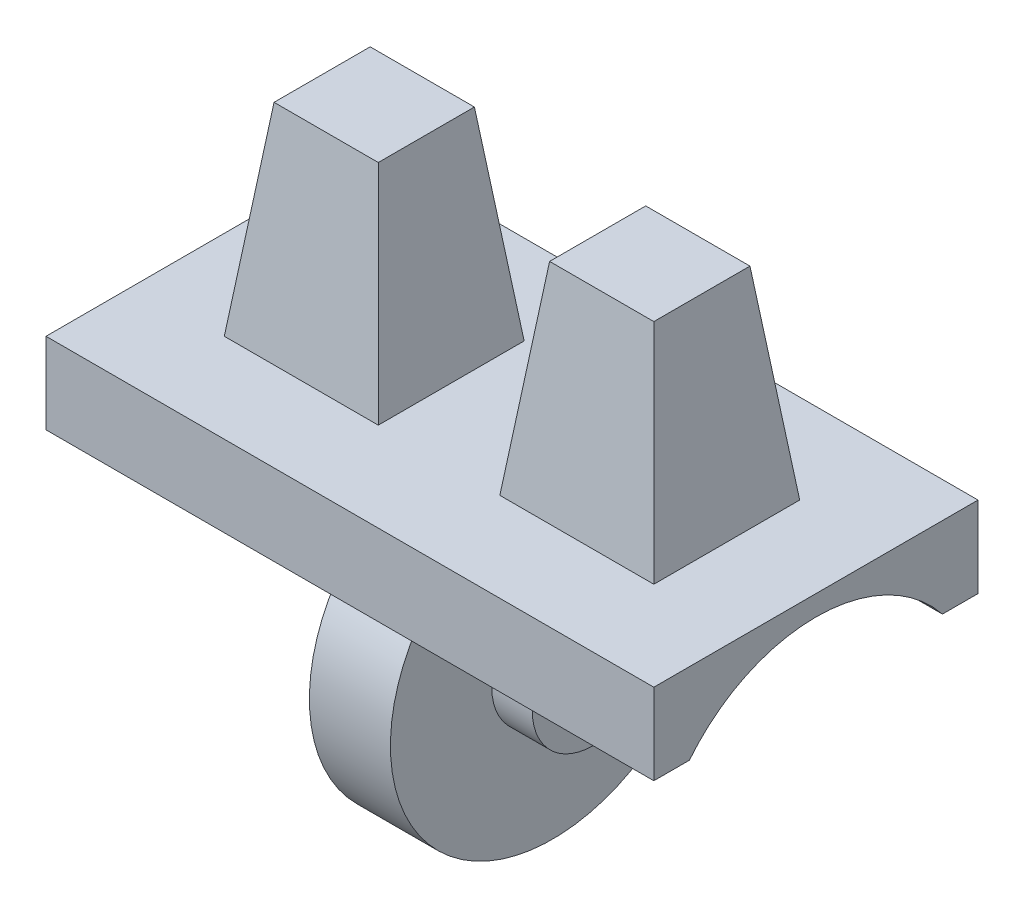
ISO-10303-21;
HEADER;
FILE_DESCRIPTION(('STEP AP214'),'2;1');
FILE_NAME('part.step','',(''),(''),'','','');
FILE_SCHEMA(('AUTOMOTIVE_DESIGN { 1 0 10303 214 1 1 1 1 }'));
ENDSEC;
DATA;
#1=APPLICATION_CONTEXT('core data for automotive mechanical design processes');
#2=APPLICATION_PROTOCOL_DEFINITION('international standard','automotive_design',2000,#1);
#3=PRODUCT_CONTEXT('',#1,'mechanical');
#4=PRODUCT('Part','Part','',(#3));
#5=PRODUCT_RELATED_PRODUCT_CATEGORY('part','',(#4));
#6=PRODUCT_DEFINITION_FORMATION('','',#4);
#7=PRODUCT_DEFINITION_CONTEXT('part definition',#1,'design');
#8=PRODUCT_DEFINITION('design','',#6,#7);
#9=PRODUCT_DEFINITION_SHAPE('','',#8);
#10=(LENGTH_UNIT() NAMED_UNIT(*) SI_UNIT(.MILLI.,.METRE.));
#11=(NAMED_UNIT(*) PLANE_ANGLE_UNIT() SI_UNIT($,.RADIAN.));
#12=(NAMED_UNIT(*) SI_UNIT($,.STERADIAN.) SOLID_ANGLE_UNIT());
#13=UNCERTAINTY_MEASURE_WITH_UNIT(LENGTH_MEASURE(1.E-05),#10,'distance_accuracy_value','');
#14=(GEOMETRIC_REPRESENTATION_CONTEXT(3) GLOBAL_UNCERTAINTY_ASSIGNED_CONTEXT((#13)) GLOBAL_UNIT_ASSIGNED_CONTEXT((#10,
#11,#12)) REPRESENTATION_CONTEXT('',''));
#15=CARTESIAN_POINT('',(0.,0.,0.));
#16=DIRECTION('',(0.,0.,1.));
#17=DIRECTION('',(1.,0.,0.));
#18=AXIS2_PLACEMENT_3D('',#15,#16,#17);
#19=CARTESIAN_POINT('',(0.,-2.5,-4.));
#20=DIRECTION('',(1.,0.,0.));
#21=DIRECTION('',(0.,0.,-1.));
#22=AXIS2_PLACEMENT_3D('',#19,#20,#21);
#23=CYLINDRICAL_SURFACE('',#22,4.);
#24=CARTESIAN_POINT('',(8.5,-2.5,-4.));
#25=DIRECTION('',(-1.,0.,0.));
#26=DIRECTION('',(0.,0.,1.));
#27=AXIS2_PLACEMENT_3D('',#24,#25,#26);
#28=CIRCLE('',#27,4.);
#29=CARTESIAN_POINT('',(8.5,0.,-0.8775010008008));
#30=VERTEX_POINT('',#29);
#31=CARTESIAN_POINT('',(8.5,0.,-7.1224989991992));
#32=VERTEX_POINT('',#31);
#33=EDGE_CURVE('E62',#30,#32,#28,.T.);
#34=ORIENTED_EDGE('',*,*,#33,.T.);
#35=DIRECTION('',(1.,0.,0.));
#36=VECTOR('',#35,1.);
#37=CARTESIAN_POINT('',(0.,0.,-7.1224989991992));
#38=LINE('',#37,#36);
#39=CARTESIAN_POINT('',(15.,0.,-7.1224989991992));
#40=VERTEX_POINT('',#39);
#41=EDGE_CURVE('E159',#32,#40,#38,.T.);
#42=ORIENTED_EDGE('',*,*,#41,.T.);
#43=CARTESIAN_POINT('',(15.,-2.5,-4.));
#44=DIRECTION('',(1.,0.,0.));
#45=DIRECTION('',(0.,0.,-1.));
#46=AXIS2_PLACEMENT_3D('',#43,#44,#45);
#47=CIRCLE('',#46,4.);
#48=CARTESIAN_POINT('',(15.,0.,-0.8775010008008));
#49=VERTEX_POINT('',#48);
#50=EDGE_CURVE('E152',#40,#49,#47,.T.);
#51=ORIENTED_EDGE('',*,*,#50,.T.);
#52=DIRECTION('',(1.,0.,0.));
#53=VECTOR('',#52,1.);
#54=CARTESIAN_POINT('',(0.,0.,-0.8775010008008));
#55=LINE('',#54,#53);
#56=EDGE_CURVE('E155',#49,#30,#55,.F.);
#57=ORIENTED_EDGE('',*,*,#56,.T.);
#58=EDGE_LOOP('',(#34,#42,#51,#57));
#59=FACE_BOUND('',#58,.T.);
#60=ADVANCED_FACE('F39',(#59),#23,.F.);
#61=CARTESIAN_POINT('',(0.,0.,0.));
#62=DIRECTION('',(0.,-1.,0.));
#63=DIRECTION('',(0.,0.,-1.));
#64=AXIS2_PLACEMENT_3D('',#61,#62,#63);
#65=PLANE('',#64);
#66=CARTESIAN_POINT('',(0.,0.,-7.1224989991992));
#67=VERTEX_POINT('',#66);
#68=CARTESIAN_POINT('',(6.5,0.,-7.1224989991992));
#69=VERTEX_POINT('',#68);
#70=EDGE_CURVE('E48',#67,#69,#38,.T.);
#71=ORIENTED_EDGE('',*,*,#70,.F.);
#72=DIRECTION('',(0.,0.,1.));
#73=VECTOR('',#72,1.);
#74=CARTESIAN_POINT('',(0.,0.,0.));
#75=LINE('',#74,#73);
#76=CARTESIAN_POINT('',(0.,0.,-8.));
#77=VERTEX_POINT('',#76);
#78=EDGE_CURVE('E262',#77,#67,#75,.T.);
#79=ORIENTED_EDGE('',*,*,#78,.F.);
#80=DIRECTION('',(-1.,0.,0.));
#81=VECTOR('',#80,1.);
#82=CARTESIAN_POINT('',(0.,0.,-8.));
#83=LINE('',#82,#81);
#84=CARTESIAN_POINT('',(15.,0.,-8.));
#85=VERTEX_POINT('',#84);
#86=EDGE_CURVE('E257',#85,#77,#83,.T.);
#87=ORIENTED_EDGE('',*,*,#86,.F.);
#88=DIRECTION('',(0.,0.,-1.));
#89=VECTOR('',#88,1.);
#90=CARTESIAN_POINT('',(15.,0.,0.));
#91=LINE('',#90,#89);
#92=EDGE_CURVE('E266',#40,#85,#91,.T.);
#93=ORIENTED_EDGE('',*,*,#92,.F.);
#94=ORIENTED_EDGE('',*,*,#41,.F.);
#95=EDGE_CURVE('E172',#69,#32,#38,.T.);
#96=ORIENTED_EDGE('',*,*,#95,.F.);
#97=EDGE_LOOP('',(#71,#79,#87,#93,#94,#96));
#98=FACE_BOUND('',#97,.T.);
#99=ADVANCED_FACE('F292',(#98),#65,.T.);
#100=CARTESIAN_POINT('',(0.,2.,0.));
#101=DIRECTION('',(0.,-1.,0.));
#102=DIRECTION('',(0.,0.,-1.));
#103=AXIS2_PLACEMENT_3D('',#100,#101,#102);
#104=PLANE('',#103);
#105=DIRECTION('',(0.,0.,1.));
#106=VECTOR('',#105,1.);
#107=CARTESIAN_POINT('',(2.2,2.,-5.8));
#108=LINE('',#107,#106);
#109=CARTESIAN_POINT('',(2.2,2.,-5.8));
#110=VERTEX_POINT('',#109);
#111=CARTESIAN_POINT('',(2.2,2.,-2.2));
#112=VERTEX_POINT('',#111);
#113=EDGE_CURVE('E203',#110,#112,#108,.T.);
#114=ORIENTED_EDGE('',*,*,#113,.F.);
#115=DIRECTION('',(-1.,0.,0.));
#116=VECTOR('',#115,1.);
#117=CARTESIAN_POINT('',(2.2,2.,-5.8));
#118=LINE('',#117,#116);
#119=CARTESIAN_POINT('',(6.,2.,-5.8));
#120=VERTEX_POINT('',#119);
#121=EDGE_CURVE('E230',#120,#110,#118,.T.);
#122=ORIENTED_EDGE('',*,*,#121,.F.);
#123=DIRECTION('',(0.,0.,-1.));
#124=VECTOR('',#123,1.);
#125=CARTESIAN_POINT('',(6.,2.,-5.8));
#126=LINE('',#125,#124);
#127=CARTESIAN_POINT('',(6.,2.,-2.2));
#128=VERTEX_POINT('',#127);
#129=EDGE_CURVE('E228',#128,#120,#126,.T.);
#130=ORIENTED_EDGE('',*,*,#129,.F.);
#131=DIRECTION('',(1.,0.,0.));
#132=VECTOR('',#131,1.);
#133=CARTESIAN_POINT('',(2.2,2.,-2.2));
#134=LINE('',#133,#132);
#135=EDGE_CURVE('E223',#112,#128,#134,.T.);
#136=ORIENTED_EDGE('',*,*,#135,.F.);
#137=EDGE_LOOP('',(#114,#122,#130,#136));
#138=FACE_BOUND('',#137,.T.);
#139=DIRECTION('',(0.,0.,1.));
#140=VECTOR('',#139,1.);
#141=CARTESIAN_POINT('',(0.,2.,0.));
#142=LINE('',#141,#140);
#143=CARTESIAN_POINT('',(0.,2.,-8.));
#144=VERTEX_POINT('',#143);
#145=CARTESIAN_POINT('',(0.,2.,0.));
#146=VERTEX_POINT('',#145);
#147=EDGE_CURVE('E251',#144,#146,#142,.T.);
#148=ORIENTED_EDGE('',*,*,#147,.T.);
#149=DIRECTION('',(1.,0.,0.));
#150=VECTOR('',#149,1.);
#151=CARTESIAN_POINT('',(0.,2.,0.));
#152=LINE('',#151,#150);
#153=CARTESIAN_POINT('',(15.,2.,0.));
#154=VERTEX_POINT('',#153);
#155=EDGE_CURVE('E259',#146,#154,#152,.T.);
#156=ORIENTED_EDGE('',*,*,#155,.T.);
#157=DIRECTION('',(0.,0.,-1.));
#158=VECTOR('',#157,1.);
#159=CARTESIAN_POINT('',(15.,2.,0.));
#160=LINE('',#159,#158);
#161=CARTESIAN_POINT('',(15.,2.,-8.));
#162=VERTEX_POINT('',#161);
#163=EDGE_CURVE('E256',#154,#162,#160,.T.);
#164=ORIENTED_EDGE('',*,*,#163,.T.);
#165=DIRECTION('',(-1.,0.,0.));
#166=VECTOR('',#165,1.);
#167=CARTESIAN_POINT('',(0.,2.,-8.));
#168=LINE('',#167,#166);
#169=EDGE_CURVE('E265',#162,#144,#168,.T.);
#170=ORIENTED_EDGE('',*,*,#169,.T.);
#171=EDGE_LOOP('',(#148,#156,#164,#170));
#172=FACE_BOUND('',#171,.T.);
#173=DIRECTION('',(-1.,0.,0.));
#174=VECTOR('',#173,1.);
#175=CARTESIAN_POINT('',(12.8,2.,-5.8));
#176=LINE('',#175,#174);
#177=CARTESIAN_POINT('',(12.8,2.,-5.8));
#178=VERTEX_POINT('',#177);
#179=CARTESIAN_POINT('',(9.,2.,-5.8));
#180=VERTEX_POINT('',#179);
#181=EDGE_CURVE('E187',#178,#180,#176,.T.);
#182=ORIENTED_EDGE('',*,*,#181,.F.);
#183=DIRECTION('',(0.,0.,-1.));
#184=VECTOR('',#183,1.);
#185=CARTESIAN_POINT('',(12.8,2.,-5.8));
#186=LINE('',#185,#184);
#187=CARTESIAN_POINT('',(12.8,2.,-2.2));
#188=VERTEX_POINT('',#187);
#189=EDGE_CURVE('E198',#188,#178,#186,.T.);
#190=ORIENTED_EDGE('',*,*,#189,.F.);
#191=DIRECTION('',(1.,0.,0.));
#192=VECTOR('',#191,1.);
#193=CARTESIAN_POINT('',(12.8,2.,-2.2));
#194=LINE('',#193,#192);
#195=CARTESIAN_POINT('',(9.,2.,-2.2));
#196=VERTEX_POINT('',#195);
#197=EDGE_CURVE('E192',#196,#188,#194,.T.);
#198=ORIENTED_EDGE('',*,*,#197,.F.);
#199=DIRECTION('',(0.,0.,1.));
#200=VECTOR('',#199,1.);
#201=CARTESIAN_POINT('',(9.,2.,-5.8));
#202=LINE('',#201,#200);
#203=EDGE_CURVE('E188',#180,#196,#202,.T.);
#204=ORIENTED_EDGE('',*,*,#203,.F.);
#205=EDGE_LOOP('',(#182,#190,#198,#204));
#206=FACE_BOUND('',#205,.T.);
#207=ADVANCED_FACE('F305',(#138,#172,#206),#104,.F.);
#208=CARTESIAN_POINT('',(0.,2.,0.));
#209=DIRECTION('',(1.,0.,0.));
#210=DIRECTION('',(0.,0.,-1.));
#211=AXIS2_PLACEMENT_3D('',#208,#209,#210);
#212=PLANE('',#211);
#213=ORIENTED_EDGE('',*,*,#78,.T.);
#214=CARTESIAN_POINT('',(0.,-2.5,-4.));
#215=DIRECTION('',(1.,0.,0.));
#216=DIRECTION('',(0.,0.,-1.));
#217=AXIS2_PLACEMENT_3D('',#214,#215,#216);
#218=CIRCLE('',#217,4.);
#219=CARTESIAN_POINT('',(0.,0.,-0.8775010008008));
#220=VERTEX_POINT('',#219);
#221=EDGE_CURVE('E182',#67,#220,#218,.T.);
#222=ORIENTED_EDGE('',*,*,#221,.T.);
#223=CARTESIAN_POINT('',(0.,0.,0.));
#224=VERTEX_POINT('',#223);
#225=EDGE_CURVE('E236',#220,#224,#75,.T.);
#226=ORIENTED_EDGE('',*,*,#225,.T.);
#227=DIRECTION('',(0.,-1.,0.));
#228=VECTOR('',#227,1.);
#229=CARTESIAN_POINT('',(0.,2.,0.));
#230=LINE('',#229,#228);
#231=EDGE_CURVE('E285',#146,#224,#230,.T.);
#232=ORIENTED_EDGE('',*,*,#231,.F.);
#233=ORIENTED_EDGE('',*,*,#147,.F.);
#234=DIRECTION('',(0.,-1.,0.));
#235=VECTOR('',#234,1.);
#236=CARTESIAN_POINT('',(0.,2.,-8.));
#237=LINE('',#236,#235);
#238=EDGE_CURVE('E264',#144,#77,#237,.T.);
#239=ORIENTED_EDGE('',*,*,#238,.T.);
#240=EDGE_LOOP('',(#213,#222,#226,#232,#233,#239));
#241=FACE_BOUND('',#240,.T.);
#242=ADVANCED_FACE('F41',(#241),#212,.F.);
#243=CARTESIAN_POINT('',(0.,2.,0.));
#244=DIRECTION('',(0.,0.,-1.));
#245=DIRECTION('',(-1.,0.,0.));
#246=AXIS2_PLACEMENT_3D('',#243,#244,#245);
#247=PLANE('',#246);
#248=DIRECTION('',(1.,0.,0.));
#249=VECTOR('',#248,1.);
#250=CARTESIAN_POINT('',(0.,0.,0.));
#251=LINE('',#250,#249);
#252=CARTESIAN_POINT('',(15.,0.,0.));
#253=VERTEX_POINT('',#252);
#254=EDGE_CURVE('E268',#224,#253,#251,.T.);
#255=ORIENTED_EDGE('',*,*,#254,.T.);
#256=DIRECTION('',(0.,-1.,0.));
#257=VECTOR('',#256,1.);
#258=CARTESIAN_POINT('',(15.,2.,0.));
#259=LINE('',#258,#257);
#260=EDGE_CURVE('E280',#154,#253,#259,.T.);
#261=ORIENTED_EDGE('',*,*,#260,.F.);
#262=ORIENTED_EDGE('',*,*,#155,.F.);
#263=ORIENTED_EDGE('',*,*,#231,.T.);
#264=EDGE_LOOP('',(#255,#261,#262,#263));
#265=FACE_BOUND('',#264,.T.);
#266=ADVANCED_FACE('F308',(#265),#247,.F.);
#267=CARTESIAN_POINT('',(15.,2.,0.));
#268=DIRECTION('',(-1.,0.,0.));
#269=DIRECTION('',(0.,0.,1.));
#270=AXIS2_PLACEMENT_3D('',#267,#268,#269);
#271=PLANE('',#270);
#272=EDGE_CURVE('E272',#253,#49,#91,.T.);
#273=ORIENTED_EDGE('',*,*,#272,.T.);
#274=ORIENTED_EDGE('',*,*,#50,.F.);
#275=ORIENTED_EDGE('',*,*,#92,.T.);
#276=DIRECTION('',(0.,-1.,0.));
#277=VECTOR('',#276,1.);
#278=CARTESIAN_POINT('',(15.,2.,-8.));
#279=LINE('',#278,#277);
#280=EDGE_CURVE('E278',#162,#85,#279,.T.);
#281=ORIENTED_EDGE('',*,*,#280,.F.);
#282=ORIENTED_EDGE('',*,*,#163,.F.);
#283=ORIENTED_EDGE('',*,*,#260,.T.);
#284=EDGE_LOOP('',(#273,#274,#275,#281,#282,#283));
#285=FACE_BOUND('',#284,.T.);
#286=ADVANCED_FACE('F289',(#285),#271,.F.);
#287=CARTESIAN_POINT('',(0.,2.,-8.));
#288=DIRECTION('',(0.,0.,1.));
#289=DIRECTION('',(1.,0.,0.));
#290=AXIS2_PLACEMENT_3D('',#287,#288,#289);
#291=PLANE('',#290);
#292=ORIENTED_EDGE('',*,*,#86,.T.);
#293=ORIENTED_EDGE('',*,*,#238,.F.);
#294=ORIENTED_EDGE('',*,*,#169,.F.);
#295=ORIENTED_EDGE('',*,*,#280,.T.);
#296=EDGE_LOOP('',(#292,#293,#294,#295));
#297=FACE_BOUND('',#296,.T.);
#298=ADVANCED_FACE('F298',(#297),#291,.F.);
#299=ORIENTED_EDGE('',*,*,#56,.F.);
#300=ORIENTED_EDGE('',*,*,#272,.F.);
#301=ORIENTED_EDGE('',*,*,#254,.F.);
#302=ORIENTED_EDGE('',*,*,#225,.F.);
#303=CARTESIAN_POINT('',(6.5,0.,-0.8775010008008));
#304=VERTEX_POINT('',#303);
#305=EDGE_CURVE('E162',#304,#220,#55,.F.);
#306=ORIENTED_EDGE('',*,*,#305,.F.);
#307=EDGE_CURVE('E156',#30,#304,#55,.F.);
#308=ORIENTED_EDGE('',*,*,#307,.F.);
#309=EDGE_LOOP('',(#299,#300,#301,#302,#306,#308));
#310=FACE_BOUND('',#309,.T.);
#311=ADVANCED_FACE('F164',(#310),#65,.T.);
#312=CARTESIAN_POINT('',(2.2,2.,-5.8));
#313=DIRECTION('',(-0.992546151641322,0.121869343405148,0.));
#314=DIRECTION('',(-0.121869343405148,-0.992546151641322,0.));
#315=AXIS2_PLACEMENT_3D('',#312,#313,#314);
#316=PLANE('',#315);
#317=ORIENTED_EDGE('',*,*,#113,.T.);
#318=DIRECTION('',(-0.120974291151355,-0.985256536015293,0.120974291151355));
#319=VECTOR('',#318,1.);
#320=CARTESIAN_POINT('',(2.2,2.,-2.2));
#321=LINE('',#320,#319);
#322=CARTESIAN_POINT('',(2.81392280451452,7.,-2.81392280451452));
#323=VERTEX_POINT('',#322);
#324=EDGE_CURVE('E231',#323,#112,#321,.T.);
#325=ORIENTED_EDGE('',*,*,#324,.F.);
#326=DIRECTION('',(0.,0.,-1.));
#327=VECTOR('',#326,1.);
#328=CARTESIAN_POINT('',(2.81392280451452,7.,-5.8));
#329=LINE('',#328,#327);
#330=CARTESIAN_POINT('',(2.81392280451452,7.,-5.18607719548548));
#331=VERTEX_POINT('',#330);
#332=EDGE_CURVE('E235',#331,#323,#329,.F.);
#333=ORIENTED_EDGE('',*,*,#332,.F.);
#334=DIRECTION('',(-0.120974291151355,-0.985256536015293,-0.120974291151355));
#335=VECTOR('',#334,1.);
#336=CARTESIAN_POINT('',(2.2,2.,-5.8));
#337=LINE('',#336,#335);
#338=EDGE_CURVE('E238',#331,#110,#337,.T.);
#339=ORIENTED_EDGE('',*,*,#338,.T.);
#340=EDGE_LOOP('',(#317,#325,#333,#339));
#341=FACE_BOUND('',#340,.T.);
#342=ADVANCED_FACE('F356',(#341),#316,.T.);
#343=CARTESIAN_POINT('',(2.2,2.,-2.2));
#344=DIRECTION('',(0.,0.121869343405148,0.992546151641322));
#345=DIRECTION('',(0.,-0.992546151641322,0.121869343405148));
#346=AXIS2_PLACEMENT_3D('',#343,#344,#345);
#347=PLANE('',#346);
#348=ORIENTED_EDGE('',*,*,#135,.T.);
#349=DIRECTION('',(0.120974291151355,-0.985256536015293,0.120974291151355));
#350=VECTOR('',#349,1.);
#351=CARTESIAN_POINT('',(5.94731479516954,2.42908655976808,-2.25268520483046));
#352=LINE('',#351,#350);
#353=CARTESIAN_POINT('',(5.38607719548548,7.,-2.81392280451452));
#354=VERTEX_POINT('',#353);
#355=EDGE_CURVE('E240',#354,#128,#352,.T.);
#356=ORIENTED_EDGE('',*,*,#355,.F.);
#357=DIRECTION('',(-1.,0.,0.));
#358=VECTOR('',#357,1.);
#359=CARTESIAN_POINT('',(2.2,7.,-2.81392280451452));
#360=LINE('',#359,#358);
#361=EDGE_CURVE('E248',#323,#354,#360,.F.);
#362=ORIENTED_EDGE('',*,*,#361,.F.);
#363=ORIENTED_EDGE('',*,*,#324,.T.);
#364=EDGE_LOOP('',(#348,#356,#362,#363));
#365=FACE_BOUND('',#364,.T.);
#366=ADVANCED_FACE('F363',(#365),#347,.T.);
#367=CARTESIAN_POINT('',(6.,2.,-5.8));
#368=DIRECTION('',(0.992546151641322,0.121869343405148,0.));
#369=DIRECTION('',(-0.121869343405148,0.992546151641322,0.));
#370=AXIS2_PLACEMENT_3D('',#367,#368,#369);
#371=PLANE('',#370);
#372=ORIENTED_EDGE('',*,*,#129,.T.);
#373=DIRECTION('',(0.120974291151355,-0.985256536015293,-0.120974291151355));
#374=VECTOR('',#373,1.);
#375=CARTESIAN_POINT('',(5.94438783934562,2.45292470197742,-5.74438783934562));
#376=LINE('',#375,#374);
#377=CARTESIAN_POINT('',(5.38607719548548,7.,-5.18607719548548));
#378=VERTEX_POINT('',#377);
#379=EDGE_CURVE('E241',#378,#120,#376,.T.);
#380=ORIENTED_EDGE('',*,*,#379,.F.);
#381=DIRECTION('',(0.,0.,1.));
#382=VECTOR('',#381,1.);
#383=CARTESIAN_POINT('',(5.38607719548548,7.,-5.8));
#384=LINE('',#383,#382);
#385=EDGE_CURVE('E252',#354,#378,#384,.F.);
#386=ORIENTED_EDGE('',*,*,#385,.F.);
#387=ORIENTED_EDGE('',*,*,#355,.T.);
#388=EDGE_LOOP('',(#372,#380,#386,#387));
#389=FACE_BOUND('',#388,.T.);
#390=ADVANCED_FACE('F362',(#389),#371,.T.);
#391=CARTESIAN_POINT('',(2.2,2.,-5.8));
#392=DIRECTION('',(0.,0.121869343405148,-0.992546151641322));
#393=DIRECTION('',(0.,0.992546151641322,0.121869343405148));
#394=AXIS2_PLACEMENT_3D('',#391,#392,#393);
#395=PLANE('',#394);
#396=ORIENTED_EDGE('',*,*,#121,.T.);
#397=ORIENTED_EDGE('',*,*,#338,.F.);
#398=DIRECTION('',(1.,0.,0.));
#399=VECTOR('',#398,1.);
#400=CARTESIAN_POINT('',(2.2,7.,-5.18607719548548));
#401=LINE('',#400,#399);
#402=EDGE_CURVE('E245',#378,#331,#401,.F.);
#403=ORIENTED_EDGE('',*,*,#402,.F.);
#404=ORIENTED_EDGE('',*,*,#379,.T.);
#405=EDGE_LOOP('',(#396,#397,#403,#404));
#406=FACE_BOUND('',#405,.T.);
#407=ADVANCED_FACE('F358',(#406),#395,.T.);
#408=CARTESIAN_POINT('',(0.,7.,0.));
#409=DIRECTION('',(0.,1.,0.));
#410=DIRECTION('',(0.,0.,1.));
#411=AXIS2_PLACEMENT_3D('',#408,#409,#410);
#412=PLANE('',#411);
#413=ORIENTED_EDGE('',*,*,#332,.T.);
#414=ORIENTED_EDGE('',*,*,#361,.T.);
#415=ORIENTED_EDGE('',*,*,#385,.T.);
#416=ORIENTED_EDGE('',*,*,#402,.T.);
#417=EDGE_LOOP('',(#413,#414,#415,#416));
#418=FACE_BOUND('',#417,.T.);
#419=ADVANCED_FACE('F341',(#418),#412,.T.);
#420=CARTESIAN_POINT('',(12.8,2.,-5.8));
#421=DIRECTION('',(0.,0.121869343405148,-0.992546151641322));
#422=DIRECTION('',(0.,0.992546151641322,0.121869343405148));
#423=AXIS2_PLACEMENT_3D('',#420,#421,#422);
#424=PLANE('',#423);
#425=ORIENTED_EDGE('',*,*,#181,.T.);
#426=DIRECTION('',(-0.120974291151355,-0.985256536015293,-0.120974291151355));
#427=VECTOR('',#426,1.);
#428=CARTESIAN_POINT('',(9.,2.,-5.8));
#429=LINE('',#428,#427);
#430=CARTESIAN_POINT('',(9.61392280451452,7.,-5.18607719548548));
#431=VERTEX_POINT('',#430);
#432=EDGE_CURVE('E197',#431,#180,#429,.T.);
#433=ORIENTED_EDGE('',*,*,#432,.F.);
#434=DIRECTION('',(1.,0.,0.));
#435=VECTOR('',#434,1.);
#436=CARTESIAN_POINT('',(12.8,7.,-5.18607719548548));
#437=LINE('',#436,#435);
#438=CARTESIAN_POINT('',(12.1860771954855,7.,-5.18607719548548));
#439=VERTEX_POINT('',#438);
#440=EDGE_CURVE('E199',#439,#431,#437,.F.);
#441=ORIENTED_EDGE('',*,*,#440,.F.);
#442=DIRECTION('',(0.120974291151355,-0.985256536015293,-0.120974291151355));
#443=VECTOR('',#442,1.);
#444=CARTESIAN_POINT('',(12.8,2.,-5.8));
#445=LINE('',#444,#443);
#446=EDGE_CURVE('E201',#439,#178,#445,.T.);
#447=ORIENTED_EDGE('',*,*,#446,.T.);
#448=EDGE_LOOP('',(#425,#433,#441,#447));
#449=FACE_BOUND('',#448,.T.);
#450=ADVANCED_FACE('F344',(#449),#424,.T.);
#451=CARTESIAN_POINT('',(9.,2.,-5.8));
#452=DIRECTION('',(-0.992546151641322,0.121869343405148,0.));
#453=DIRECTION('',(-0.121869343405148,-0.992546151641322,0.));
#454=AXIS2_PLACEMENT_3D('',#451,#452,#453);
#455=PLANE('',#454);
#456=ORIENTED_EDGE('',*,*,#203,.T.);
#457=DIRECTION('',(-0.120974291151355,-0.985256536015293,0.120974291151355));
#458=VECTOR('',#457,1.);
#459=CARTESIAN_POINT('',(9.05561216065438,2.45292470197742,-2.25561216065438));
#460=LINE('',#459,#458);
#461=CARTESIAN_POINT('',(9.61392280451452,7.,-2.81392280451452));
#462=VERTEX_POINT('',#461);
#463=EDGE_CURVE('E204',#462,#196,#460,.T.);
#464=ORIENTED_EDGE('',*,*,#463,.F.);
#465=DIRECTION('',(0.,0.,-1.));
#466=VECTOR('',#465,1.);
#467=CARTESIAN_POINT('',(9.61392280451452,7.,-5.8));
#468=LINE('',#467,#466);
#469=EDGE_CURVE('E218',#431,#462,#468,.F.);
#470=ORIENTED_EDGE('',*,*,#469,.F.);
#471=ORIENTED_EDGE('',*,*,#432,.T.);
#472=EDGE_LOOP('',(#456,#464,#470,#471));
#473=FACE_BOUND('',#472,.T.);
#474=ADVANCED_FACE('F345',(#473),#455,.T.);
#475=CARTESIAN_POINT('',(12.8,2.,-2.2));
#476=DIRECTION('',(0.,0.121869343405148,0.992546151641322));
#477=DIRECTION('',(0.,-0.992546151641322,0.121869343405148));
#478=AXIS2_PLACEMENT_3D('',#475,#476,#477);
#479=PLANE('',#478);
#480=ORIENTED_EDGE('',*,*,#197,.T.);
#481=DIRECTION('',(0.120974291151355,-0.985256536015293,0.120974291151355));
#482=VECTOR('',#481,1.);
#483=CARTESIAN_POINT('',(12.7473147951695,2.42908655976808,-2.25268520483046));
#484=LINE('',#483,#482);
#485=CARTESIAN_POINT('',(12.1860771954855,7.,-2.81392280451452));
#486=VERTEX_POINT('',#485);
#487=EDGE_CURVE('E206',#486,#188,#484,.T.);
#488=ORIENTED_EDGE('',*,*,#487,.F.);
#489=DIRECTION('',(-1.,0.,0.));
#490=VECTOR('',#489,1.);
#491=CARTESIAN_POINT('',(12.8,7.,-2.81392280451452));
#492=LINE('',#491,#490);
#493=EDGE_CURVE('E216',#462,#486,#492,.F.);
#494=ORIENTED_EDGE('',*,*,#493,.F.);
#495=ORIENTED_EDGE('',*,*,#463,.T.);
#496=EDGE_LOOP('',(#480,#488,#494,#495));
#497=FACE_BOUND('',#496,.T.);
#498=ADVANCED_FACE('F336',(#497),#479,.T.);
#499=CARTESIAN_POINT('',(12.8,2.,-5.8));
#500=DIRECTION('',(0.992546151641322,0.121869343405148,0.));
#501=DIRECTION('',(-0.121869343405148,0.992546151641322,0.));
#502=AXIS2_PLACEMENT_3D('',#499,#500,#501);
#503=PLANE('',#502);
#504=ORIENTED_EDGE('',*,*,#189,.T.);
#505=ORIENTED_EDGE('',*,*,#446,.F.);
#506=DIRECTION('',(0.,0.,1.));
#507=VECTOR('',#506,1.);
#508=CARTESIAN_POINT('',(12.1860771954855,7.,-5.8));
#509=LINE('',#508,#507);
#510=EDGE_CURVE('E209',#486,#439,#509,.F.);
#511=ORIENTED_EDGE('',*,*,#510,.F.);
#512=ORIENTED_EDGE('',*,*,#487,.T.);
#513=EDGE_LOOP('',(#504,#505,#511,#512));
#514=FACE_BOUND('',#513,.T.);
#515=ADVANCED_FACE('F333',(#514),#503,.T.);
#516=CARTESIAN_POINT('',(0.,7.,0.));
#517=DIRECTION('',(0.,1.,0.));
#518=DIRECTION('',(0.,0.,1.));
#519=AXIS2_PLACEMENT_3D('',#516,#517,#518);
#520=PLANE('',#519);
#521=ORIENTED_EDGE('',*,*,#440,.T.);
#522=ORIENTED_EDGE('',*,*,#469,.T.);
#523=ORIENTED_EDGE('',*,*,#493,.T.);
#524=ORIENTED_EDGE('',*,*,#510,.T.);
#525=EDGE_LOOP('',(#521,#522,#523,#524));
#526=FACE_BOUND('',#525,.T.);
#527=ADVANCED_FACE('F328',(#526),#520,.T.);
#528=ORIENTED_EDGE('',*,*,#70,.T.);
#529=CARTESIAN_POINT('',(6.5,-2.5,-4.));
#530=DIRECTION('',(-1.,0.,0.));
#531=DIRECTION('',(0.,0.,1.));
#532=AXIS2_PLACEMENT_3D('',#529,#530,#531);
#533=CIRCLE('',#532,4.);
#534=EDGE_CURVE('E54',#304,#69,#533,.T.);
#535=ORIENTED_EDGE('',*,*,#534,.F.);
#536=ORIENTED_EDGE('',*,*,#305,.T.);
#537=ORIENTED_EDGE('',*,*,#221,.F.);
#538=EDGE_LOOP('',(#528,#535,#536,#537));
#539=FACE_BOUND('',#538,.T.);
#540=ADVANCED_FACE('F319',(#539),#23,.F.);
#541=CARTESIAN_POINT('',(6.5,-2.5,-4.));
#542=DIRECTION('',(1.,0.,0.));
#543=DIRECTION('',(0.,0.,-1.));
#544=AXIS2_PLACEMENT_3D('',#541,#542,#543);
#545=CYLINDRICAL_SURFACE('',#544,4.);
#546=ORIENTED_EDGE('',*,*,#95,.T.);
#547=EDGE_CURVE('E175',#32,#30,#28,.T.);
#548=ORIENTED_EDGE('',*,*,#547,.T.);
#549=ORIENTED_EDGE('',*,*,#307,.T.);
#550=EDGE_CURVE('E177',#69,#304,#533,.T.);
#551=ORIENTED_EDGE('',*,*,#550,.F.);
#552=EDGE_LOOP('',(#546,#548,#549,#551));
#553=FACE_BOUND('',#552,.T.);
#554=ADVANCED_FACE('F173',(#553),#545,.T.);
#555=CARTESIAN_POINT('',(6.5,-2.5,-4.));
#556=DIRECTION('',(-1.,0.,0.));
#557=DIRECTION('',(0.,0.,1.));
#558=AXIS2_PLACEMENT_3D('',#555,#556,#557);
#559=PLANE('',#558);
#560=CARTESIAN_POINT('',(6.5,-2.5,-4.));
#561=DIRECTION('',(-1.,0.,0.));
#562=DIRECTION('',(0.,0.,1.));
#563=AXIS2_PLACEMENT_3D('',#560,#561,#562);
#564=CIRCLE('',#563,1.5);
#565=CARTESIAN_POINT('',(6.5,-2.5,-2.5));
#566=VERTEX_POINT('',#565);
#567=EDGE_CURVE('E43',#566,#566,#564,.F.);
#568=ORIENTED_EDGE('',*,*,#567,.T.);
#569=EDGE_LOOP('',(#568));
#570=FACE_BOUND('',#569,.T.);
#571=ORIENTED_EDGE('',*,*,#534,.T.);
#572=ORIENTED_EDGE('',*,*,#550,.T.);
#573=EDGE_LOOP('',(#571,#572));
#574=FACE_BOUND('',#573,.T.);
#575=ADVANCED_FACE('F332',(#570,#574),#559,.T.);
#576=CARTESIAN_POINT('',(8.5,-2.5,-4.));
#577=DIRECTION('',(-1.,0.,0.));
#578=DIRECTION('',(0.,0.,1.));
#579=AXIS2_PLACEMENT_3D('',#576,#577,#578);
#580=PLANE('',#579);
#581=CARTESIAN_POINT('',(8.5,-2.5,-4.));
#582=DIRECTION('',(-1.,0.,0.));
#583=DIRECTION('',(0.,0.,1.));
#584=AXIS2_PLACEMENT_3D('',#581,#582,#583);
#585=CIRCLE('',#584,1.5);
#586=CARTESIAN_POINT('',(8.5,-2.5,-2.5));
#587=VERTEX_POINT('',#586);
#588=EDGE_CURVE('E11',#587,#587,#585,.F.);
#589=ORIENTED_EDGE('',*,*,#588,.F.);
#590=EDGE_LOOP('',(#589));
#591=FACE_BOUND('',#590,.T.);
#592=ORIENTED_EDGE('',*,*,#33,.F.);
#593=ORIENTED_EDGE('',*,*,#547,.F.);
#594=EDGE_LOOP('',(#592,#593));
#595=FACE_BOUND('',#594,.T.);
#596=ADVANCED_FACE('F178',(#591,#595),#580,.F.);
#597=CARTESIAN_POINT('',(9.5,-2.5,-4.));
#598=DIRECTION('',(-1.,0.,0.));
#599=DIRECTION('',(0.,0.,1.));
#600=AXIS2_PLACEMENT_3D('',#597,#598,#599);
#601=CYLINDRICAL_SURFACE('',#600,1.5);
#602=CARTESIAN_POINT('',(9.5,-2.5,-4.));
#603=DIRECTION('',(1.,0.,0.));
#604=DIRECTION('',(0.,0.,-1.));
#605=AXIS2_PLACEMENT_3D('',#602,#603,#604);
#606=CIRCLE('',#605,1.5);
#607=CARTESIAN_POINT('',(9.5,-2.5,-5.5));
#608=VERTEX_POINT('',#607);
#609=EDGE_CURVE('E176',#608,#608,#606,.T.);
#610=ORIENTED_EDGE('',*,*,#609,.F.);
#611=EDGE_LOOP('',(#610));
#612=FACE_BOUND('',#611,.T.);
#613=ORIENTED_EDGE('',*,*,#588,.T.);
#614=EDGE_LOOP('',(#613));
#615=FACE_BOUND('',#614,.T.);
#616=ADVANCED_FACE('F475',(#612,#615),#601,.T.);
#617=CARTESIAN_POINT('',(9.5,-2.5,-4.));
#618=DIRECTION('',(1.,0.,0.));
#619=DIRECTION('',(0.,0.,-1.));
#620=AXIS2_PLACEMENT_3D('',#617,#618,#619);
#621=PLANE('',#620);
#622=ORIENTED_EDGE('',*,*,#609,.T.);
#623=EDGE_LOOP('',(#622));
#624=FACE_BOUND('',#623,.T.);
#625=ADVANCED_FACE('F484',(#624),#621,.T.);
#626=CARTESIAN_POINT('',(5.5,-2.5,-4.));
#627=DIRECTION('',(1.,0.,0.));
#628=DIRECTION('',(0.,0.,-1.));
#629=AXIS2_PLACEMENT_3D('',#626,#627,#628);
#630=CYLINDRICAL_SURFACE('',#629,1.5);
#631=ORIENTED_EDGE('',*,*,#567,.F.);
#632=EDGE_LOOP('',(#631));
#633=FACE_BOUND('',#632,.T.);
#634=CARTESIAN_POINT('',(5.5,-2.5,-4.));
#635=DIRECTION('',(-1.,0.,0.));
#636=DIRECTION('',(0.,0.,1.));
#637=AXIS2_PLACEMENT_3D('',#634,#635,#636);
#638=CIRCLE('',#637,1.5);
#639=CARTESIAN_POINT('',(5.5,-2.5,-2.5));
#640=VERTEX_POINT('',#639);
#641=EDGE_CURVE('E519',#640,#640,#638,.T.);
#642=ORIENTED_EDGE('',*,*,#641,.F.);
#643=EDGE_LOOP('',(#642));
#644=FACE_BOUND('',#643,.T.);
#645=ADVANCED_FACE('F491',(#633,#644),#630,.T.);
#646=CARTESIAN_POINT('',(5.5,-2.5,-4.));
#647=DIRECTION('',(-1.,0.,0.));
#648=DIRECTION('',(0.,0.,1.));
#649=AXIS2_PLACEMENT_3D('',#646,#647,#648);
#650=PLANE('',#649);
#651=ORIENTED_EDGE('',*,*,#641,.T.);
#652=EDGE_LOOP('',(#651));
#653=FACE_BOUND('',#652,.T.);
#654=ADVANCED_FACE('F505',(#653),#650,.T.);
#655=CLOSED_SHELL('',(#60,#99,#207,#242,#266,#286,#298,#311,#342,#366,#390,#407,#419,#450,#474,
#498,#515,#527,#540,#554,#575,#596,#616,#625,#645,#654));
#656=MANIFOLD_SOLID_BREP('B2',#655);
#657=ADVANCED_BREP_SHAPE_REPRESENTATION('',(#18,#656),#14);
#658=SHAPE_DEFINITION_REPRESENTATION(#9,#657);
ENDSEC;
END-ISO-10303-21;
